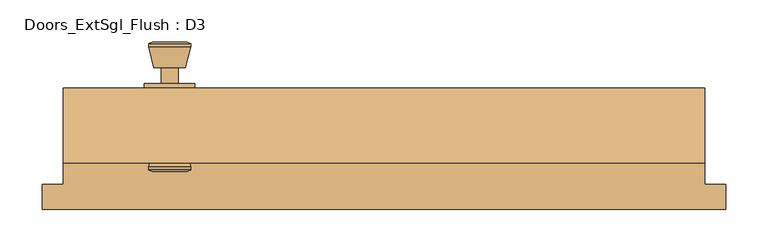
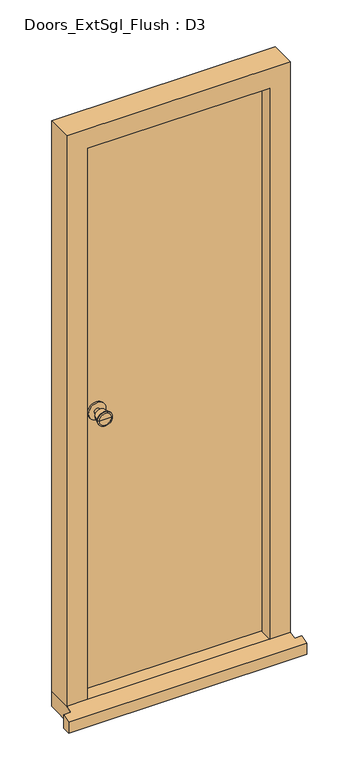
"""IFC4 building model written with IfcOpenShell, lengths in millimetres: door geometry, Doors_ExtSgl_Flush : D3."""

from ifc_helpers import new_model, si_unit, point, frame, frame_2d, origin, place, context, project, spatial, polyline, circle_curve, trimmed, segment, composite_curve, outline, extrude, faceted_brep, source, transform, mapped, element, save
from ifc_brep_helpers import plane_surface, cylinder_surface, revolved_surface, advanced_brep


def doors_extsgl_flush_d3_352cde1d(model_context):
    return source(origin(), model_context, "Body", "SolidModel", [
        advanced_brep(
        [(-254.5, 43.8, 1050.0), (-264.5, 43.8, 1050.0), (-244.5, 43.8, 1050.0), (-234.0241324, 92.8, 1050.0), (-274.9758676, 92.8, 1050.0), (-254.5, 92.8, 1050.0), (-229.5, 90.9721319, 1050.0), (-279.5, 90.9721319, 1050.0), (-229.5, 87.5084537, 1050.0), (-279.5, 87.5084537, 1050.0), (-235.863764, 62.8, 1050.0), (-273.136236, 62.8, 1050.0), (-244.5, 62.8, 1050.0), (-264.5, 62.8, 1050.0)],
        [
            (0, 1),
            (1, 2, circle_curve(frame((-254.5, 43.8, 1050.0), z_axis=(0.0, -1.0, 0.0), x_axis=(-1.0, 0.0, 0.0)), 10.0)),
            (2, 0),
            (2, 1, circle_curve(frame((-254.5, 43.8, 1050.0), z_axis=(0.0, -1.0, 0.0), x_axis=(-1.0, 0.0, 0.0)), 10.0)),
            (3, 4, circle_curve(frame((-254.5, 92.8, 1050.0), z_axis=(0.0, 1.0, 0.0), x_axis=(-1.0, 0.0, 0.0)), 20.4758676)),
            (4, 5),
            (5, 3),
            (4, 3, circle_curve(frame((-254.5, 92.8, 1050.0), z_axis=(0.0, 1.0, 0.0), x_axis=(-1.0, 0.0, 0.0)), 20.4758676)),
            (6, 7, circle_curve(frame((-254.5, 90.9721319, 1050.0), z_axis=(0.0, 1.0, 0.0), x_axis=(-1.0, 0.0, 0.0)), 25.0)),
            (7, 4),
            (3, 6),
            (7, 6, circle_curve(frame((-254.5, 90.9721319, 1050.0), z_axis=(0.0, 1.0, 0.0), x_axis=(-1.0, 0.0, 0.0)), 25.0)),
            (8, 9, circle_curve(frame((-254.5, 87.5084537, 1050.0), z_axis=(0.0, 1.0, 0.0), x_axis=(-1.0, 0.0, 0.0)), 25.0)),
            (9, 7),
            (6, 8),
            (9, 8, circle_curve(frame((-254.5, 87.5084537, 1050.0), z_axis=(0.0, 1.0, 0.0), x_axis=(-1.0, 0.0, 0.0)), 25.0)),
            (10, 11, circle_curve(frame((-254.5, 62.8, 1050.0), z_axis=(0.0, 1.0, 0.0), x_axis=(-1.0, 0.0, 0.0)), 18.636236)),
            (11, 9),
            (8, 10),
            (11, 10, circle_curve(frame((-254.5, 62.8, 1050.0), z_axis=(0.0, 1.0, 0.0), x_axis=(-1.0, 0.0, 0.0)), 18.636236)),
            (12, 13, circle_curve(frame((-254.5, 62.8, 1050.0), z_axis=(0.0, 1.0, 0.0), x_axis=(-1.0, 0.0, 0.0)), 10.0)),
            (13, 11),
            (10, 12),
            (13, 12, circle_curve(frame((-254.5, 62.8, 1050.0), z_axis=(0.0, 1.0, 0.0), x_axis=(-1.0, 0.0, 0.0)), 10.0)),
            (1, 13),
            (12, 2),
        ],
        [
            plane_surface(frame((-254.5, 43.8, 1050.0), z_axis=(0.0, -1.0, 0.0), x_axis=(-1.0, 0.0, 0.0))),
            plane_surface(frame((-254.5, 92.8, 1050.0), z_axis=(0.0, 1.0, 0.0), x_axis=(-1.0, 0.0, 0.0))),
            revolved_surface(polyline([(-274.9758676, 92.8, 1050.0), (-279.5, 90.9721319, 1050.0)]), (-254.5, 43.8, 1050.0), (0.0, -1.0, 0.0)),
            cylinder_surface(frame((-254.5, 43.8, 1050.0), z_axis=(0.0, -1.0, 0.0), x_axis=(-1.0, 0.0, 0.0)), 25.0),
            revolved_surface(polyline([(-279.5, 87.5084537, 1050.0), (-273.136236, 62.8, 1050.0)]), (-254.5, 43.8, 1050.0), (0.0, -1.0, 0.0)),
            plane_surface(frame((-254.5, 62.8, 1050.0), z_axis=(0.0, -1.0, 0.0), x_axis=(-1.0, 0.0, 0.0))),
            cylinder_surface(frame((-254.5, 43.8, 1050.0), z_axis=(0.0, -1.0, 0.0), x_axis=(-1.0, 0.0, 0.0)), 10.0),
        ],
        [
            (0, [[1, 2, 3]]),
            (0, [[-3, 4, -1]]),
            (1, [[5, 6, 7]]),
            (1, [[8, -7, -6]]),
            (2, [[9, 10, -5, 11]]),
            (2, [[12, -11, -8, -10]]),
            (3, [[13, 14, -9, 15]]),
            (3, [[16, -15, -12, -14]]),
            (4, [[17, 18, -13, 19]]),
            (4, [[20, -19, -16, -18]]),
            (5, [[21, 22, -17, 23]]),
            (5, [[24, -23, -20, -22]]),
            (6, [[-2, 25, -21, 26]]),
            (6, [[-4, -26, -24, -25]]),
        ],
    ),
        extrude(outline(composite_curve([segment(trimmed(circle_curve(frame_2d((1050.0, -254.5)), 30.0), [point((1050.0, -284.5))], [point((1050.0, -224.5))], False, "CARTESIAN"), True, "CONTINUOUS"), segment(trimmed(circle_curve(frame_2d((1050.0, -254.5)), 30.0), [point((1050.0, -224.5))], [point((1050.0, -284.5))], False, "CARTESIAN"), True, "CONTINUOUS")], self_intersect=False)), frame((0.0, 37.8, 0.0), z_axis=(0.0, 1.0, 0.0), x_axis=(0.0, 0.0, 1.0)), (0.0, 0.0, 1.0), 6.0),
        advanced_brep(
        [(-254.5, -12.2, 1050.0), (-244.5, -12.2, 1050.0), (-264.5, -12.2, 1050.0), (-234.0241324, -61.2, 1050.0), (-254.5, -61.2, 1050.0), (-274.9758676, -61.2, 1050.0), (-229.5, -59.3721319, 1050.0), (-279.5, -59.3721319, 1050.0), (-229.5, -55.9084537, 1050.0), (-279.5, -55.9084537, 1050.0), (-235.863764, -31.2, 1050.0), (-273.136236, -31.2, 1050.0), (-244.5, -31.2, 1050.0), (-264.5, -31.2, 1050.0)],
        [
            (0, 1),
            (1, 2, circle_curve(frame((-254.5, -12.2, 1050.0), z_axis=(0.0, 1.0, 0.0), x_axis=(-1.0, 0.0, 0.0)), 10.0)),
            (2, 0),
            (2, 1, circle_curve(frame((-254.5, -12.2, 1050.0), z_axis=(0.0, 1.0, 0.0), x_axis=(-1.0, 0.0, 0.0)), 10.0)),
            (3, 4),
            (4, 5),
            (5, 3, circle_curve(frame((-254.5, -61.2, 1050.0), z_axis=(0.0, -1.0, 0.0), x_axis=(-1.0, 0.0, 0.0)), 20.4758676)),
            (3, 5, circle_curve(frame((-254.5, -61.2, 1050.0), z_axis=(0.0, -1.0, 0.0), x_axis=(-1.0, 0.0, 0.0)), 20.4758676)),
            (6, 3),
            (5, 7),
            (7, 6, circle_curve(frame((-254.5, -59.3721319, 1050.0), z_axis=(0.0, -1.0, 0.0), x_axis=(-1.0, 0.0, 0.0)), 25.0)),
            (6, 7, circle_curve(frame((-254.5, -59.3721319, 1050.0), z_axis=(0.0, -1.0, 0.0), x_axis=(-1.0, 0.0, 0.0)), 25.0)),
            (8, 6),
            (7, 9),
            (9, 8, circle_curve(frame((-254.5, -55.9084537, 1050.0), z_axis=(0.0, -1.0, 0.0), x_axis=(-1.0, 0.0, 0.0)), 25.0)),
            (8, 9, circle_curve(frame((-254.5, -55.9084537, 1050.0), z_axis=(0.0, -1.0, 0.0), x_axis=(-1.0, 0.0, 0.0)), 25.0)),
            (10, 8),
            (9, 11),
            (11, 10, circle_curve(frame((-254.5, -31.2, 1050.0), z_axis=(0.0, -1.0, 0.0), x_axis=(-1.0, 0.0, 0.0)), 18.636236)),
            (10, 11, circle_curve(frame((-254.5, -31.2, 1050.0), z_axis=(0.0, -1.0, 0.0), x_axis=(-1.0, 0.0, 0.0)), 18.636236)),
            (12, 10),
            (11, 13),
            (13, 12, circle_curve(frame((-254.5, -31.2, 1050.0), z_axis=(0.0, -1.0, 0.0), x_axis=(-1.0, 0.0, 0.0)), 10.0)),
            (12, 13, circle_curve(frame((-254.5, -31.2, 1050.0), z_axis=(0.0, -1.0, 0.0), x_axis=(-1.0, 0.0, 0.0)), 10.0)),
            (1, 12),
            (13, 2),
        ],
        [
            plane_surface(frame((-254.5, -12.2, 1050.0), z_axis=(0.0, 1.0, 0.0), x_axis=(-1.0, 0.0, 0.0))),
            plane_surface(frame((-254.5, -61.2, 1050.0), z_axis=(0.0, -1.0, 0.0), x_axis=(-1.0, 0.0, 0.0))),
            revolved_surface(polyline([(-274.9758676, -61.2, 1050.0), (-279.5, -59.3721319, 1050.0)]), (-254.5, -12.2, 1050.0), (0.0, 1.0, 0.0)),
            cylinder_surface(frame((-254.5, -12.2, 1050.0), z_axis=(0.0, 1.0, 0.0), x_axis=(-1.0, 0.0, 0.0)), 25.0),
            revolved_surface(polyline([(-279.5, -55.9084537, 1050.0), (-273.136236, -31.2, 1050.0)]), (-254.5, -12.2, 1050.0), (0.0, 1.0, 0.0)),
            plane_surface(frame((-254.5, -31.2, 1050.0), z_axis=(0.0, 1.0, 0.0), x_axis=(-1.0, 0.0, 0.0))),
            cylinder_surface(frame((-254.5, -12.2, 1050.0), z_axis=(0.0, 1.0, 0.0), x_axis=(-1.0, 0.0, 0.0)), 10.0),
        ],
        [
            (0, [[1, 2, 3]]),
            (0, [[-3, 4, -1]]),
            (1, [[5, 6, 7]]),
            (1, [[-6, -5, 8]]),
            (2, [[9, -7, 10, 11]]),
            (2, [[-10, -8, -9, 12]]),
            (3, [[13, -11, 14, 15]]),
            (3, [[-14, -12, -13, 16]]),
            (4, [[17, -15, 18, 19]]),
            (4, [[-18, -16, -17, 20]]),
            (5, [[21, -19, 22, 23]]),
            (5, [[-22, -20, -21, 24]]),
            (6, [[25, -23, 26, -2]]),
            (6, [[-26, -24, -25, -4]]),
        ],
    ),
        extrude(outline(composite_curve([segment(trimmed(circle_curve(frame_2d((1050.0, -254.5)), 30.0), [point((1050.0, -284.5))], [point((1050.0, -224.5))], False, "CARTESIAN"), True, "CONTINUOUS"), segment(trimmed(circle_curve(frame_2d((1050.0, -254.5)), 30.0), [point((1050.0, -224.5))], [point((1050.0, -284.5))], False, "CARTESIAN"), True, "CONTINUOUS")], self_intersect=False)), frame((0.0, -12.2, 0.0), z_axis=(0.0, 1.0, 0.0), x_axis=(0.0, 0.0, 1.0)), (0.0, 0.0, 1.0), 6.0),
        faceted_brep([(310.5, -51.2, 54.5), (310.5, -9.2, 54.5), (332.5, -9.2, 54.5), (332.5, 37.8, 54.5), (381.0, 37.8, 54.5), (381.0, -51.2, 54.5), (381.0, -51.2, 2110.0), (-381.0, -51.2, 2110.0), (-381.0, -51.2, 54.5), (-310.5, -51.2, 54.5), (-310.5, -51.2, 2039.5), (310.5, -51.2, 2039.5), (381.0, 37.8, 2110.0), (332.5, 37.8, 2061.5), (-332.5, 37.8, 2061.5), (-332.5, 37.8, 54.5), (-381.0, 37.8, 54.5), (-381.0, 37.8, 2110.0), (332.5, -9.2, 2061.5), (310.5, -9.2, 2039.5), (-310.5, -9.2, 2039.5), (-310.5, -9.2, 54.5), (-332.5, -9.2, 54.5), (-332.5, -9.2, 2061.5)], [[[0, 1, 2, 3, 4, 5]], [[5, 6, 7, 8, 9, 10, 11, 0]], [[4, 12, 6, 5]], [[3, 13, 14, 15, 16, 17, 12, 4]], [[2, 18, 13, 3]], [[1, 19, 20, 21, 22, 23, 18, 2]], [[0, 11, 19, 1]], [[10, 9, 21, 20]], [[9, 8, 16, 15, 22, 21]], [[17, 16, 8, 7]], [[23, 22, 15, 14]], [[12, 17, 7, 6]], [[18, 23, 14, 13]], [[11, 10, 20, 19]]]),
        extrude(outline(polyline([(329.5, 37.8), (329.5, -6.2), (-330.4250294, -6.2), (-330.4250294, 37.8), (329.5, 37.8)])), frame((0.0, 0.0, 58.5), z_axis=(0.0, 0.0, 1.0), x_axis=(1.0, 0.0, 0.0)), (0.0, 0.0, 1.0), 2000.0),
        faceted_brep([(406.0, -106.2, 0.0), (406.0, -76.2, 0.0), (406.0, -76.2, 47.2703282), (406.0, -106.2, 38.5947221), (-406.0, -106.2, 38.5947221), (-406.0, -76.2, 47.2703282), (-406.0, -76.2, 0.0), (-406.0, -106.2, 0.0), (-381.0, -76.2, 0.0), (-381.0, 37.8, 0.0), (381.0, 37.8, 0.0), (381.0, -76.2, 0.0), (381.0, -76.2, 47.2703282), (381.0, -51.2, 54.5), (-381.0, -51.2, 54.5), (-381.0, -76.2, 47.2703282), (381.0, 37.8, 54.5), (-381.0, 37.8, 54.5)], [[[0, 1, 2, 3]], [[4, 5, 6, 7]], [[7, 6, 8, 9, 10, 11, 1, 0]], [[3, 4, 7, 0]], [[3, 2, 12, 13, 14, 15, 5, 4]], [[14, 13, 16, 17]], [[17, 16, 10, 9]], [[15, 14, 17, 9, 8]], [[8, 6, 5, 15]], [[11, 10, 16, 13, 12]], [[12, 2, 1, 11]]]),
    ])


if __name__ == "__main__":
    model = new_model("IFC4")
    model_context = context("Model", 3, world=origin())
    ifc_project = project(units=[si_unit("LENGTHUNIT", "METRE", prefix="MILLI")], contexts=[model_context])
    site = spatial("IfcSite", under=ifc_project)
    building = spatial("IfcBuilding", under=site)
    placement = place(None, origin())
    doors_extsgl_flush_d3_shape = doors_extsgl_flush_d3_352cde1d(model_context)
    element("IfcDoor", 1, ObjectType="Doors_ExtSgl_Flush : D3", at=placement, inside=building, context=model_context, shape_type="MappedRepresentation", body=[
        mapped(doors_extsgl_flush_d3_shape, transform((0.0, 0.0, 0.0), x_axis=(1.0, 0.0, 0.0), y_axis=(0.0, 1.0, 0.0), z_axis=(0.0, 0.0, 1.0))),
    ])
    save(model, "model.ifc")

# Revit data of these elements
# Type "Doors_ExtSgl_Flush : D3"
#   Type Mark = "51"
#   Type Comments = "External Single"
#   Operation = "SingleSwingRight"
#   Construction Type Id = "MDOOR"
#   Keynote = "L20"
#   Analytic Construction = "Metal"
#   Wrap Layers (Int) from Ext = 177.5 mm
#   Wrap Layers (Ext) from Ext = 102.5 mm
#   Thickness = 44 mm
#   Rough Width = 762 mm
#   Rough Height = 2110 mm
#   O/A Frame Width = 64 mm
#   Heat Transfer Coefficient (U) = 3.7021 W/(m²·K)
#   Handle Z Distance = 1050 mm
#   FrameWidth = 42 mm
#   FrameOffset - External = 25 mm
#   FrameDepth = 89 mm
#   Door Panel Width = 659 mm
#   Door Panel Thickness = 44 mm
#   Door Panel Height = 2000 mm
#   Cill Thickness = 54.5 mm
#   Cill Projection = 30 mm
#   Handle X Distance = 75 mm
#   Height = 2110 mm
#   Structural Tolerance = 6.5 mm
#   Tolerance = 3 mm
#   Undercut = 4 mm
#   Width = 762 mm
#   Cill Extension = 25 mm
#   Cavity Closer Width = 50 mm
#   Cavity Closer Offset from Ext = 102.5 mm
#   Cavity Closer Depth = 85 mm
#   Vis - Ironmongery = yes
#   Vis - Cavity Closers = yes
#   Define Thermal Properties by = 1
#   Function = 1
#   Material Door = Door - Panel
#   Material Frame = Door - Frame/Mullion
#   Material Ironmongery = Door - Handle
#   Visual Light Transmittance = 0
#   Solar Heat Gain Coefficient = 0
#   Wall Closure = (empty or 0)
# Element 1 (IfcDoor, "Doors_ExtSgl_Flush : D3")
#   Materials on its faces: "Door - Handle", "Door - Frame/Mullion", "Door - Panel"
# Materials
#   "Door - Panel": class "Wood", colour RGB 210 159 95, transparency 0, Keynote = "L20", Cost = 0
#   "Door - Frame/Mullion": class "Wood", colour RGB 212 179 113, transparency 0, Keynote = "L20", Cost = 0
#   "Door - Handle": colour RGB 0 0 0, transparency 0, Keynote = "P21", Cost = 0
